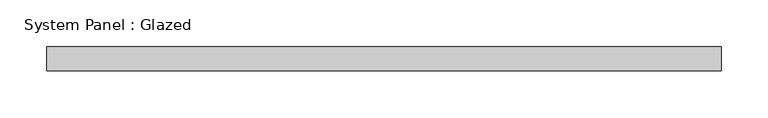
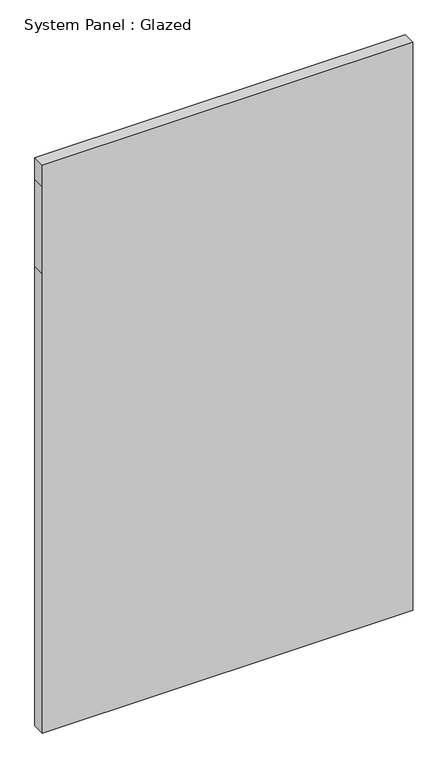
"""IFC4 building model written with IfcOpenShell, lengths in millimetres: plate geometry, System Panel : Glazed."""

from ifc_helpers import new_model, si_unit, frame, origin, place, context, project, spatial, polyline, outline, extrude, source, transform, mapped, element, save


def system_panel_glazed_9ec27a3c(model_context):
    return source(origin(), model_context, "Body", "SweptSolid", [
        extrude(outline(polyline([(0.0, -358.775), (0.0, 358.775), (941.116916, 358.775), (1118.916916, 358.775), (1163.366916, 358.775), (1163.366916, -358.775), (1118.916916, -358.775), (941.116916, -358.775), (0.0, -358.775)])), frame((0.0, 19.05, 0.0), z_axis=(0.0, 1.0, 0.0), x_axis=(0.0, 0.0, 1.0)), (0.0, 0.0, 1.0), 25.4),
    ])


if __name__ == "__main__":
    model = new_model("IFC4")
    model_context = context("Model", 3, world=origin())
    ifc_project = project(units=[si_unit("LENGTHUNIT", "METRE", prefix="MILLI")], contexts=[model_context])
    site = spatial("IfcSite", under=ifc_project)
    building = spatial("IfcBuilding", under=site)
    placement = place(None, origin())
    system_panel_glazed_shape = system_panel_glazed_9ec27a3c(model_context)
    element("IfcPlate", 1, ObjectType="System Panel : Glazed", at=placement, inside=building, context=model_context, shape_type="MappedRepresentation", body=[
        mapped(system_panel_glazed_shape, transform((0.0, 0.0, 0.0), x_axis=(1.0, 0.0, 0.0), y_axis=(0.0, 1.0, 0.0), z_axis=(0.0, 0.0, 1.0))),
    ])
    save(model, "model.ifc")

# Revit data of these elements
# Type "System Panel : Glazed"
#   Construction Type Id = "GSP4R"
#   Analytic Construction = "1/8 in Pilkington single glazing"
#   Visual Light Transmittance = 0.9
#   Solar Heat Gain Coefficient = 0.86
#   Heat Transfer Coefficient (U) = 1.18115 BTU/(h·ft²·°F)
#   Define Thermal Properties by = 1
# Element 1 (IfcPlate, "System Panel : Glazed")
#   Materials on its faces: "Glass"
# Materials
#   "Glass": class "Glass", colour RGB 0 128 192, transparency 0.75, Description = "Soda Lime Glass", Cost = 0
